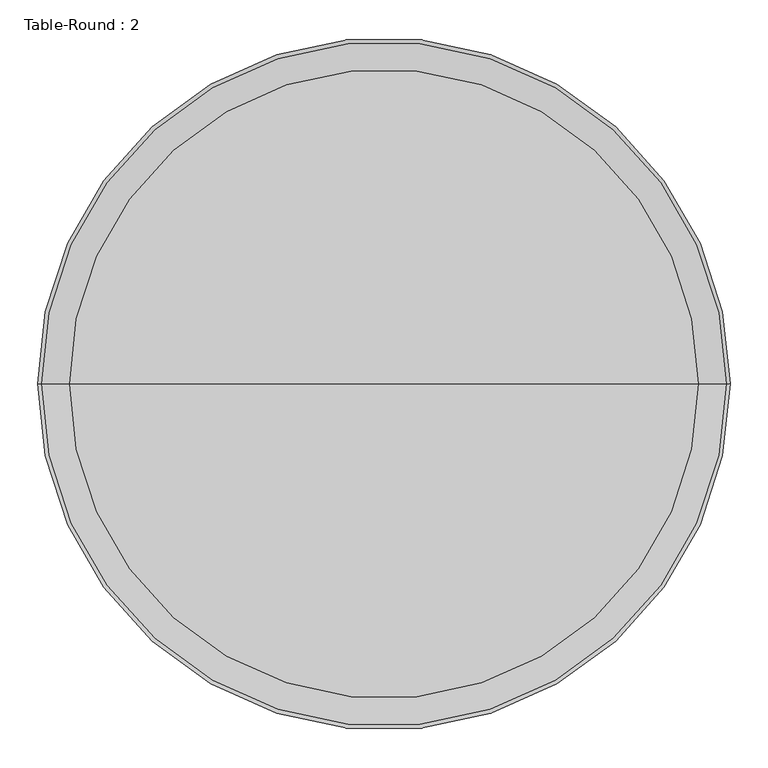
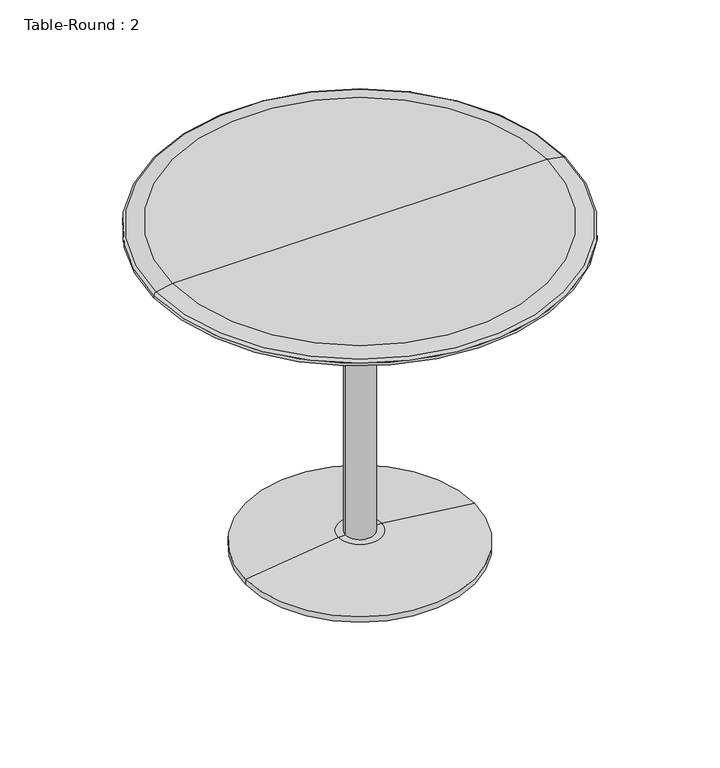
"""IFC4 building model written with IfcOpenShell, lengths in millimetres: furniture geometry, Table-Round : 2."""

from ifc_helpers import new_model, si_unit, point, frame, origin, origin_2d, place, context, project, spatial, polyline, circle_curve, ellipse_curve, trimmed, segment, composite_curve, outline, extrude, source, transform, mapped, element, save
from ifc_brep_helpers import plane_surface, cylinder_surface, revolved_surface, advanced_brep


def table_round_2_c80d6d9c(model_context):
    return source(origin(), model_context, "Body", "SolidModel", [
        extrude(outline(composite_curve([segment(trimmed(circle_curve(origin_2d(), 31.75), [point((-31.75, 0.0))], [point((31.75, 0.0))], False, "CARTESIAN"), True, "CONTINUOUS"), segment(trimmed(circle_curve(origin_2d(), 31.75), [point((31.75, 0.0))], [point((-31.75, 0.0))], False, "CARTESIAN"), True, "CONTINUOUS")], self_intersect=False)), frame((0.0, 0.0, 38.1), z_axis=(0.0, 0.0, 1.0), x_axis=(1.0, 0.0, 0.0)), (0.0, 0.0, 1.0), 704.85),
        advanced_brep(
        [(0.0, 0.0, 742.95), (-457.2, 0.0, 742.95), (457.2, 0.0, 742.95), (415.3011364, 0.0, 762.0), (-415.3011364, 0.0, 762.0), (0.0, 0.0, 762.0), (451.9526659, 0.0, 755.5373465), (-451.9526659, 0.0, 755.5373465), (457.2, 0.0, 749.2838172), (-457.2, 0.0, 749.2838172)],
        [
            (0, 1),
            (1, 2, circle_curve(frame((0.0, 0.0, 742.95), z_axis=(0.0, 0.0, -1.0), x_axis=(-1.0, 0.0, 0.0)), 457.2)),
            (2, 0),
            (2, 1, circle_curve(frame((0.0, 0.0, 742.95), z_axis=(0.0, 0.0, -1.0), x_axis=(-1.0, 0.0, 0.0)), 457.2)),
            (3, 4, circle_curve(frame((0.0, 0.0, 762.0), z_axis=(0.0, 0.0, 1.0), x_axis=(-1.0, 0.0, 0.0)), 415.3011364)),
            (4, 5),
            (5, 3),
            (4, 3, circle_curve(frame((0.0, 0.0, 762.0), z_axis=(0.0, 0.0, 1.0), x_axis=(-1.0, 0.0, 0.0)), 415.3011364)),
            (6, 7, circle_curve(frame((0.0, 0.0, 755.5373465), z_axis=(0.0, 0.0, 1.0), x_axis=(-1.0, 0.0, 0.0)), 451.9526659)),
            (7, 4),
            (3, 6),
            (7, 6, circle_curve(frame((0.0, 0.0, 755.5373465), z_axis=(0.0, 0.0, 1.0), x_axis=(-1.0, 0.0, 0.0)), 451.9526659)),
            (8, 9, circle_curve(frame((0.0, 0.0, 749.2838172), z_axis=(0.0, 0.0, 1.0), x_axis=(-1.0, 0.0, 0.0)), 457.2)),
            (9, 7, circle_curve(frame((-450.85, 0.0, 749.2838172), z_axis=(0.0, 1.0, 0.0), x_axis=(1.0, 0.0, 0.0)), 6.35)),
            (6, 8, circle_curve(frame((450.85, 0.0, 749.2838172), z_axis=(0.0, 1.0, 0.0), x_axis=(-1.0, 0.0, 0.0)), 6.35)),
            (9, 8, circle_curve(frame((0.0, 0.0, 749.2838172), z_axis=(0.0, 0.0, 1.0), x_axis=(-1.0, 0.0, 0.0)), 457.2)),
            (1, 9),
            (8, 2),
        ],
        [
            plane_surface(frame((0.0, 0.0, 742.95), z_axis=(0.0, 0.0, -1.0), x_axis=(-1.0, 0.0, 0.0))),
            plane_surface(frame((0.0, 0.0, 762.0), z_axis=(0.0, 0.0, 1.0), x_axis=(-1.0, 0.0, 0.0))),
            revolved_surface(polyline([(-415.3011364, 0.0, 762.0), (-451.9526659, 0.0, 755.5373465)]), (0.0, 0.0, 838.2), (0.0, 0.0, -1.0)),
            revolved_surface(trimmed(ellipse_curve(frame((-450.85, 0.0, 749.2838172), z_axis=(0.0, -1.0, 0.0), x_axis=(1.0, 0.0, 0.0)), 6.35, 6.35), [point((-451.9526659, 0.0, 755.5373465))], [point((-457.2, 0.0, 749.2838172))], True, "CARTESIAN"), (0.0, 0.0, 838.2), (0.0, 0.0, -1.0)),
            cylinder_surface(frame((0.0, 0.0, 838.2), z_axis=(0.0, 0.0, -1.0), x_axis=(-1.0, 0.0, 0.0)), 457.2),
        ],
        [
            (0, [[1, 2, 3]]),
            (0, [[-3, 4, -1]]),
            (1, [[5, 6, 7]]),
            (1, [[8, -7, -6]]),
            (2, [[9, 10, -5, 11]]),
            (2, [[12, -11, -8, -10]]),
            (3, [[13, 14, -9, 15]]),
            (3, [[16, -15, -12, -14]]),
            (4, [[-2, 17, -13, 18]]),
            (4, [[-4, -18, -16, -17]]),
        ],
    ),
        advanced_brep(
        [(0.0, 0.0, 0.0), (-254.0, 0.0, 0.0), (254.0, 0.0, 0.0), (47.625, 0.0, 38.1), (-47.625, 0.0, 38.1), (0.0, 0.0, 38.1), (254.0, 0.0, 12.7), (-254.0, 0.0, 12.7)],
        [
            (0, 1),
            (1, 2, circle_curve(frame((0.0, 0.0, 0.0), z_axis=(0.0, 0.0, -1.0), x_axis=(-1.0, 0.0, 0.0)), 254.0)),
            (2, 0),
            (2, 1, circle_curve(frame((0.0, 0.0, 0.0), z_axis=(0.0, 0.0, -1.0), x_axis=(-1.0, 0.0, 0.0)), 254.0)),
            (3, 4, circle_curve(frame((0.0, 0.0, 38.1), z_axis=(0.0, 0.0, 1.0), x_axis=(-1.0, 0.0, 0.0)), 47.625)),
            (4, 5),
            (5, 3),
            (4, 3, circle_curve(frame((0.0, 0.0, 38.1), z_axis=(0.0, 0.0, 1.0), x_axis=(-1.0, 0.0, 0.0)), 47.625)),
            (6, 7, circle_curve(frame((0.0, 0.0, 12.7), z_axis=(0.0, 0.0, 1.0), x_axis=(-1.0, 0.0, 0.0)), 254.0)),
            (7, 4),
            (3, 6),
            (7, 6, circle_curve(frame((0.0, 0.0, 12.7), z_axis=(0.0, 0.0, 1.0), x_axis=(-1.0, 0.0, 0.0)), 254.0)),
            (1, 7),
            (6, 2),
        ],
        [
            plane_surface(frame((0.0, 0.0, 0.0), z_axis=(0.0, 0.0, -1.0), x_axis=(-1.0, 0.0, 0.0))),
            plane_surface(frame((0.0, 0.0, 38.1), z_axis=(0.0, 0.0, 1.0), x_axis=(-1.0, 0.0, 0.0))),
            revolved_surface(polyline([(-47.625, 0.0, 38.1), (-254.0, 0.0, 12.7)]), (0.0, 0.0, 215.9), (0.0, 0.0, -1.0)),
            cylinder_surface(frame((0.0, 0.0, 215.9), z_axis=(0.0, 0.0, -1.0), x_axis=(-1.0, 0.0, 0.0)), 254.0),
        ],
        [
            (0, [[1, 2, 3]]),
            (0, [[-3, 4, -1]]),
            (1, [[5, 6, 7]]),
            (1, [[8, -7, -6]]),
            (2, [[9, 10, -5, 11]]),
            (2, [[12, -11, -8, -10]]),
            (3, [[-2, 13, -9, 14]]),
            (3, [[-4, -14, -12, -13]]),
        ],
    ),
    ])


if __name__ == "__main__":
    model = new_model("IFC4")
    model_context = context("Model", 3, world=origin())
    ifc_project = project(units=[si_unit("LENGTHUNIT", "METRE", prefix="MILLI")], contexts=[model_context])
    site = spatial("IfcSite", under=ifc_project)
    building = spatial("IfcBuilding", under=site)
    placement = place(None, origin())
    table_round_2_shape = table_round_2_c80d6d9c(model_context)
    element("IfcFurniture", 1, ObjectType="Table-Round : 2", at=placement, inside=building, context=model_context, shape_type="MappedRepresentation", body=[
        mapped(table_round_2_shape, transform((0.0, 0.0, 0.0), x_axis=(1.0, 0.0, 0.0), y_axis=(0.0, 1.0, 0.0), z_axis=(0.0, 0.0, 1.0))),
    ])
    save(model, "model.ifc")

# Revit data of these elements
# Type "Table-Round : 2"
#   Assembly Code = "E2020200"
#   Base Radius = 0' - 10"
#   Height = 2' - 6"
#   Radius = 1' - 6"
#   Base Material = Steel, Chrome Plated
#   Top Material = Birch
#   Default Elevation = 0
# Element 1 (IfcFurniture, "Table-Round : 2")
#   Materials on its faces: "Steel, Chrome Plated", "Birch"
# Materials
#   "Steel, Chrome Plated": class "Metal", colour RGB 17 17 17, transparency 0, Description = "Chromiuim plated steel", Cost = 0
#   "Birch": class "Wood", colour RGB 224 178 126, transparency 0, Description = "Betula Alleghaniensis", Cost = 0
